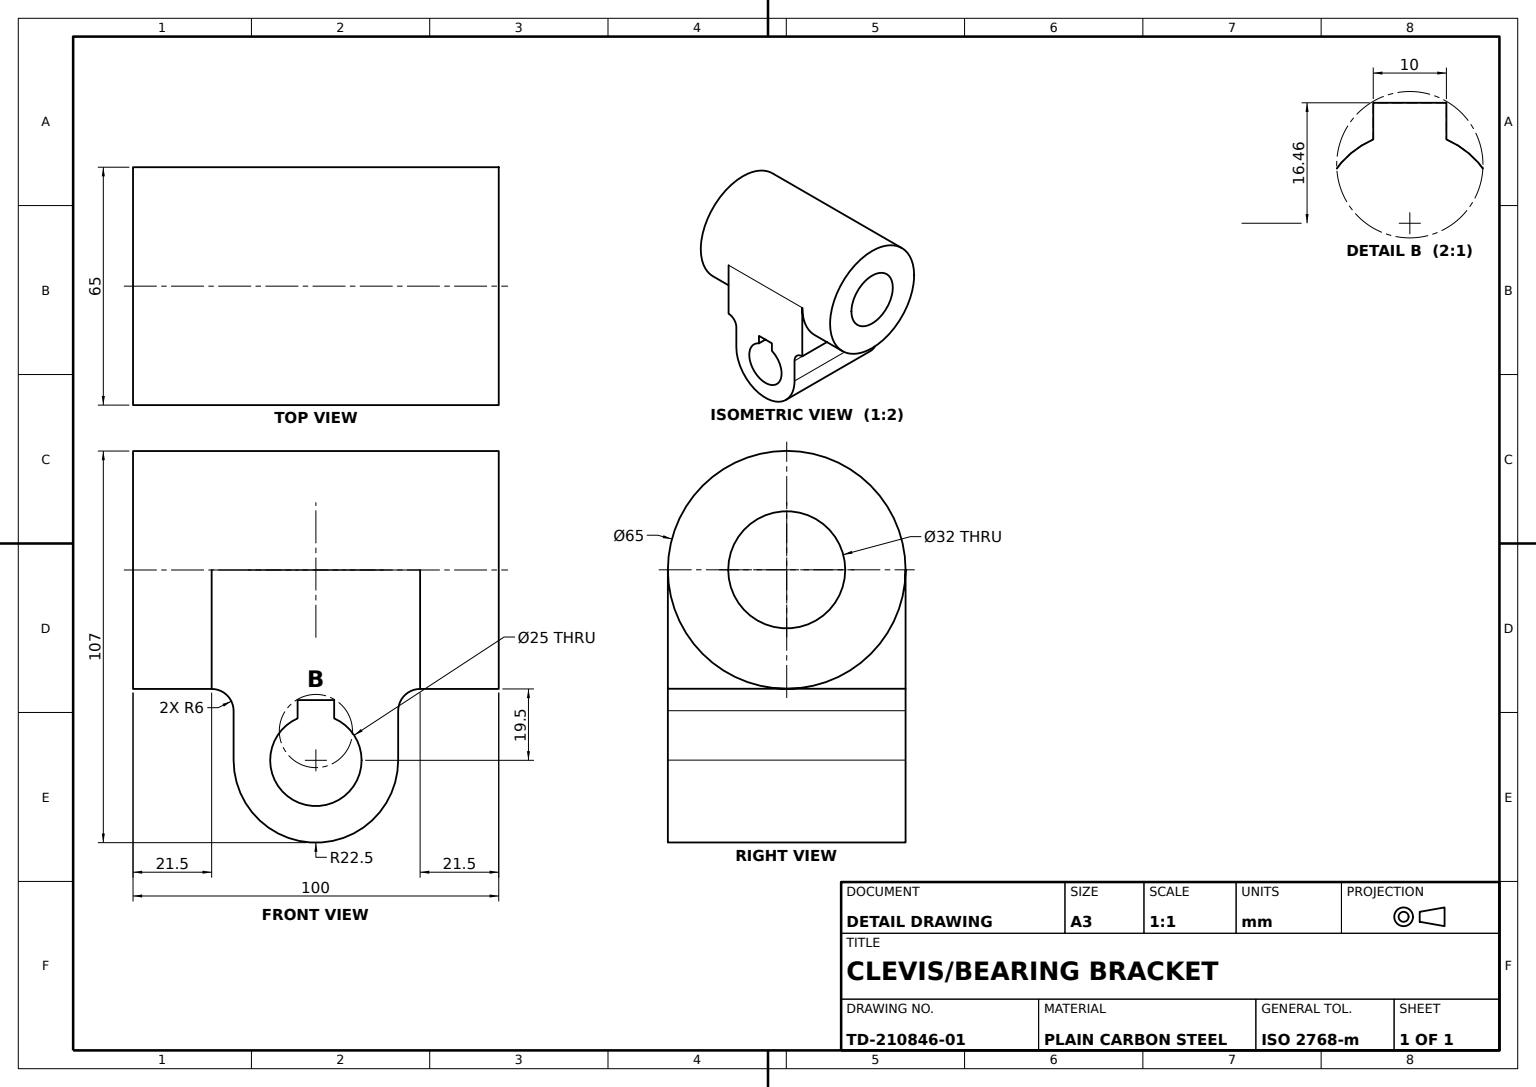
SolidWorks part; units mm, degrees
material "Plain Carbon Steel"
ref_plane "Front Plane" through (0, 0, 0) normal (0, 0, 1) x (1, 0, 0)
ref_plane "Top Plane" through (0, 0, 0) normal (0, 1, 0) x (1, 0, 0)
ref_plane "Right Plane" through (0, 0, 0) normal (1, 0, 0) x (0, 0, -1)
sketch "Sleeve Profile Ø65-Ø32" plane through (0, 0, 0) normal (1, 0, 0) x (0, 0, -1)
  circle A0 centre (0, 0) radius 32.5
  circle A1 centre (0, 0) radius 16
  dimension "D1" = 65
  dimension "D2" = 32
extrude "Sleeve Ø65x100" add sketch "Sleeve Profile Ø65-Ø32" along normal mid plane 100
sketch "Bracket Web Profile" plane through (0, 0, 0) normal (0, 0, 1) x (1, 0, 0)
  line L0 (-28.5, 0) -> (28.5, 0)
  line L1 (0, 0) -> (0, -52)
  line L3 (-5, -40.5436) -> (-5, -35.5436)
  line L4 (-5, -35.5436) -> (5, -35.5436)
  line L5 (5, -40.5436) -> (5, -35.5436)
  line L7 (22.5, -52) -> (22.5, -14.0112)
  line L8 (-50, -32.5) -> (50, -32.5)
  line L9 (28.5, -32.5) -> (28.5, 0)
  line L10 (28.5, 0) -> (23.078, -11.4419)
  line L11 (-28.5, -32.5) -> (-28.5, 0)
  line L12 (-28.5, 0) -> (-23.078, -11.4419)
  line L13 (-22.5, -52) -> (-22.5, -14.0112)
  line L15 (0, 0) -> (-28.5, 0)
  line L16 (-28.5, 0) -> (28.5, 0)
  arc A0 (-5, -40.5436) -> (5, -40.5436) centre (0, -52) ccw
  arc A1 (-22.5, -52) -> (22.5, -52) centre (0, -52) ccw
  arc A2 (28.5, -32.5) -> (22.5, -38.5) centre (28.5, -38.5) ccw
  arc A3 (22.5, -14.0112) -> (23.078, -11.4419) centre (28.5, -14.0112) cw
  arc A4 (-28.5, -32.5) -> (-22.5, -38.5) centre (-28.5, -38.5) cw
  arc A5 (-22.5, -14.0112) -> (-23.078, -11.4419) centre (-28.5, -14.0112) ccw
  dimension "D1" = 25
  dimension "D2" = 45
  dimension "D7" = 12
  dimension "D8" = 6
  dimension "D3" = 52
  dimension "D4" = 10
  dimension "D5" = 5
  dimension "D6" = 5
  dimension "D9" = 154.645
extrude "Bracket Web" add sketch "Bracket Web Profile" along normal mid plane 65 separate body
sketch "Side Rail Profile" plane through (0, 0, 32.5) normal (0, 0, 1) x (1, 0, 0)
  line L0 (-28.5, 0) -> (28.5, 0)
  line L1 (-28.5, -32.5) -> (-28.5, 0)
  line L2 (-22.5, -52) -> (-22.5, -11.1266)
  line L4 (-23.4471, -7.8911) -> (-28.5, 0)
  line L5 (23.4471, -7.8911) -> (28.5, 0)
  line L6 (22.5, -52) -> (22.5, -11.1266)
  line L7 (28.5, -32.5) -> (28.5, 0)
  arc A0 (-22.5, -11.1266) -> (-23.4471, -7.8911) centre (-28.5, -11.1266) ccw
  arc A1 (-22.5, -38.5) -> (-28.5, -32.5) centre (-28.5, -38.5) ccw
  arc A2 (22.5, -38.5) -> (28.5, -32.5) centre (28.5, -38.5) cw
  arc A3 (22.5, -11.1266) -> (23.4471, -7.8911) centre (28.5, -11.1266) cw
  circle A4 centre (0, -52) radius 22.5
  line M2 (28.5, -32.5) -> (-28.5, -32.5)
  arc M3 (-28.5, -32.5) -> (-22.5, -38.5) centre (-28.5, -38.5) cw
  line M4 (-22.5, -38.5) -> (-22.5, -52)
  arc M5 (-22.5, -52) -> (22.5, -52) centre (0, -52) ccw
  line M6 (22.5, -52) -> (22.5, -38.5)
  arc M7 (22.5, -38.5) -> (28.5, -32.5) centre (28.5, -38.5) cw
  line M8 (-5, -40.5436) -> (-5, -35.5436)
  line M9 (-5, -35.5436) -> (5, -35.5436)
  line M10 (5, -35.5436) -> (5, -40.5436)
  arc M11 (5, -40.5436) -> (-5, -40.5436) centre (0, -52) cw
  dimension "D1" = 6
  dimension "D2" = 45
  dimension "D3" = 45.9471
  dimension "D4" = 32.5
  dimension "D5" = 19.5
extrude "Side Rails" add sketch "Side Rail Profile" against normal blind 65 contours L2 M3 M2 | L2 A0 L4 L1 M2 | A4 L6 A3 L5 L0 L4 A0 L2 M2 | A3 L6 L7 L5 M2 | A4 L6 M6 M2 | L6 M7 M2 | A4 L2 M2 M4 | A4 M5 M2 M11 M8 M9 M10 | A4 M2
sketch "Lug Hole Profile" plane through (50, 0, 0) normal (1, 0, 0) x (0, 0, -1)
  circle A0 centre (0, 0) radius 16
  dimension "D1" = 32
extrude "Lug Hole Through" cut sketch "Lug Hole Profile" against normal blind 255
